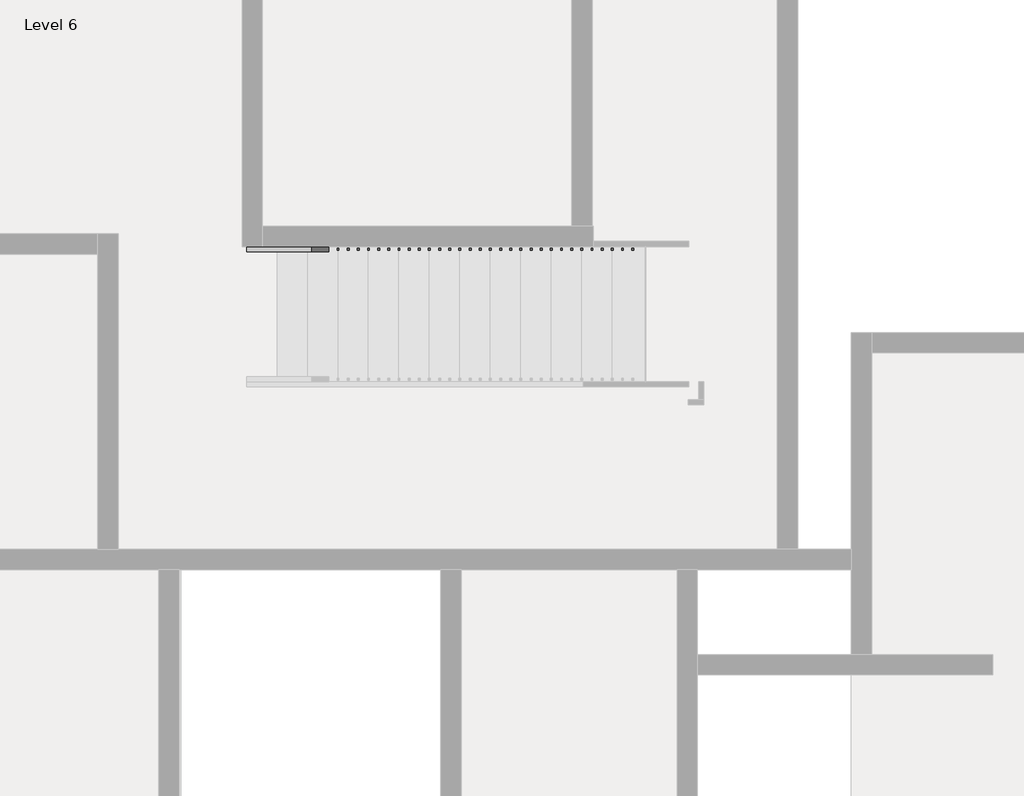
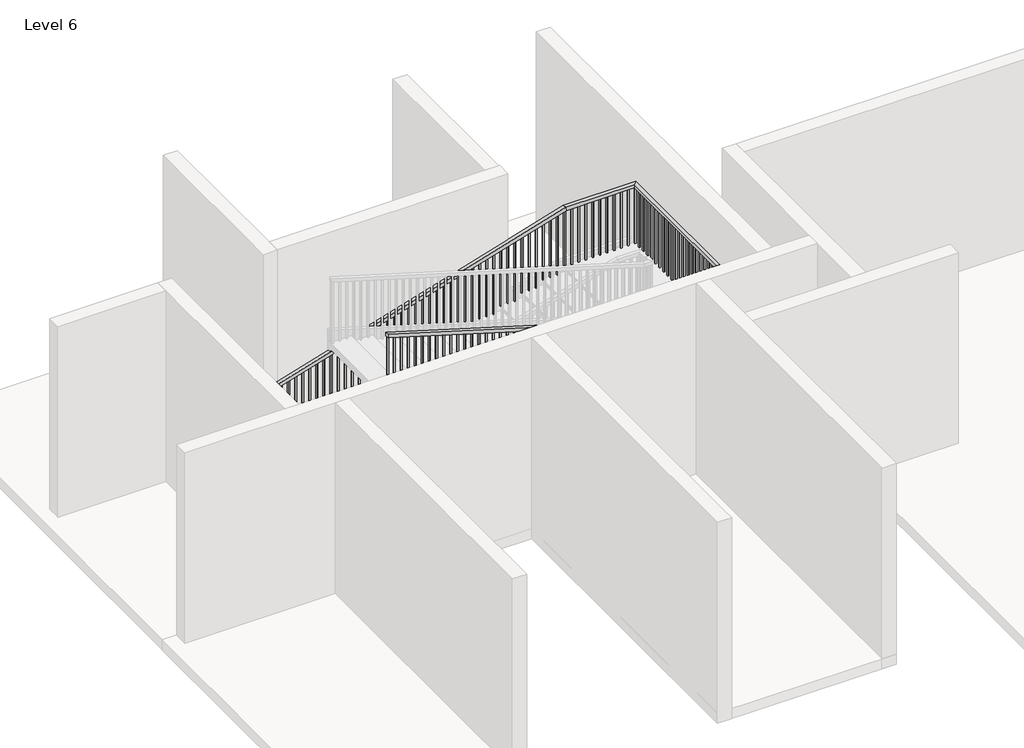
# One storey, part 10 of 14: 1 railing.
"""IFC4 building model written with IfcOpenShell, lengths in millimetres."""

from ifc_helpers import new_model, si_unit, frame, origin, place, context, project, spatial, polyline, outline, extrude, faceted_brep, element, save

model = new_model("IFC4")

# Units and contexts
model_context = context("Model", 3, world=origin())
ifc_project = project(units=[si_unit("LENGTHUNIT", "METRE", prefix="MILLI")], contexts=[model_context])

# Site, building, storey
site = spatial("IfcSite", under=ifc_project)
building = spatial("IfcBuilding", under=site)
storey = spatial("IfcBuildingStorey", under=building, Name="Level 6", Elevation=15240.0)

# Railing
placement = place(None, origin())
element("IfcRailing", 1, ObjectType="Handrail - Rectangular", at=placement, inside=storey, context=model_context, shape_type="SolidModel", body=[
    faceted_brep([(-5254.0891351, 12506.0715905, 16245.84), (-5254.0891351, 12506.0715905, 16192.8032429), (-5254.0891351, 12455.2715905, 16192.8032429), (-5254.0891351, 12455.2715905, 16245.84), (-986.8891351, 12506.0715905, 17526.0), (-979.4332782, 12506.0715905, 17475.2), (-979.4332782, 12455.2715905, 17475.2), (-986.8891351, 12455.2715905, 17526.0), (54.5108649, 12506.0715905, 17526.0), (54.5108649, 12506.0715905, 17475.2), (3.7108649, 12455.2715905, 17475.2), (3.7108649, 12455.2715905, 17526.0), (54.5108649, 9478.4949943, 17526.0), (54.5108649, 9478.4949943, 17475.2), (3.7108649, 9529.2949943, 17475.2), (3.7108649, 9529.2949943, 17526.0), (-682.0891351, 9478.4949943, 17526.0), (-689.544992, 9478.4949943, 17475.2), (-689.544992, 9529.2949943, 17475.2), (-682.0891351, 9529.2949943, 17526.0), (-5254.0891351, 9478.4949943, 18897.6), (-5254.0891351, 9529.2949943, 18897.6), (-5254.0891351, 9529.2949943, 18844.5632429), (-5254.0891351, 9478.4949943, 18844.5632429)], [[[0, 1, 2, 3]], [[1, 0, 4, 5]], [[2, 1, 5, 6]], [[3, 2, 6, 7]], [[0, 3, 7, 4]], [[5, 4, 8, 9]], [[6, 5, 9, 10]], [[7, 6, 10, 11]], [[4, 7, 11, 8]], [[9, 8, 12, 13]], [[10, 9, 13, 14]], [[11, 10, 14, 15]], [[8, 11, 15, 12]], [[13, 12, 16, 17]], [[14, 13, 17, 18]], [[15, 14, 18, 19]], [[12, 15, 19, 16]], [[20, 21, 22, 23]], [[17, 16, 20, 23]], [[18, 17, 23, 22]], [[19, 18, 22, 21]], [[16, 19, 21, 20]]]),
    extrude(outline(polyline([(18816.9407429, -5162.0141351), (17891.76, -5162.0141351), (17891.76, -5142.9641351), (18811.2257429, -5142.9641351), (18816.9407429, -5162.0141351)])), frame((0.0, 9494.3699943, 0.0), z_axis=(0.0, 1.0, 0.0), x_axis=(0.0, 0.0, 1.0)), (0.0, 0.0, 1.0), 19.05),
    extrude(outline(polyline([(18786.4607429, -5060.4141351), (17891.76, -5060.4141351), (17891.76, -5041.3641351), (18780.7457429, -5041.3641351), (18786.4607429, -5060.4141351)])), frame((0.0, 9494.3699943, 0.0), z_axis=(0.0, 1.0, 0.0), x_axis=(0.0, 0.0, 1.0)), (0.0, 0.0, 1.0), 19.05),
    extrude(outline(polyline([(18755.9807429, -4958.8141351), (17891.76, -4958.8141351), (17891.76, -4939.7641351), (18750.2657429, -4939.7641351), (18755.9807429, -4958.8141351)])), frame((0.0, 9494.3699943, 0.0), z_axis=(0.0, 1.0, 0.0), x_axis=(0.0, 0.0, 1.0)), (0.0, 0.0, 1.0), 19.05),
    extrude(outline(polyline([(18725.5007429, -4857.2141351), (17800.32, -4857.2141351), (17800.32, -4838.1641351), (18719.7857429, -4838.1641351), (18725.5007429, -4857.2141351)])), frame((0.0, 9494.3699943, 0.0), z_axis=(0.0, 1.0, 0.0), x_axis=(0.0, 0.0, 1.0)), (0.0, 0.0, 1.0), 19.05),
    extrude(outline(polyline([(18695.0207429, -4755.6141351), (17800.32, -4755.6141351), (17800.32, -4736.5641351), (18689.3057429, -4736.5641351), (18695.0207429, -4755.6141351)])), frame((0.0, 9494.3699943, 0.0), z_axis=(0.0, 1.0, 0.0), x_axis=(0.0, 0.0, 1.0)), (0.0, 0.0, 1.0), 19.05),
    extrude(outline(polyline([(18664.5407429, -4654.0141351), (17800.32, -4654.0141351), (17800.32, -4634.9641351), (18658.8257429, -4634.9641351), (18664.5407429, -4654.0141351)])), frame((0.0, 9494.3699943, 0.0), z_axis=(0.0, 1.0, 0.0), x_axis=(0.0, 0.0, 1.0)), (0.0, 0.0, 1.0), 19.05),
    extrude(outline(polyline([(18634.0607429, -4552.4141351), (17708.88, -4552.4141351), (17708.88, -4533.3641351), (18628.3457429, -4533.3641351), (18634.0607429, -4552.4141351)])), frame((0.0, 9494.3699943, 0.0), z_axis=(0.0, 1.0, 0.0), x_axis=(0.0, 0.0, 1.0)), (0.0, 0.0, 1.0), 19.05),
    extrude(outline(polyline([(18603.5807429, -4450.8141351), (17708.88, -4450.8141351), (17708.88, -4431.7641351), (18597.8657429, -4431.7641351), (18603.5807429, -4450.8141351)])), frame((0.0, 9494.3699943, 0.0), z_axis=(0.0, 1.0, 0.0), x_axis=(0.0, 0.0, 1.0)), (0.0, 0.0, 1.0), 19.05),
    extrude(outline(polyline([(18573.1007429, -4349.2141351), (17708.88, -4349.2141351), (17708.88, -4330.1641351), (18567.3857429, -4330.1641351), (18573.1007429, -4349.2141351)])), frame((0.0, 9494.3699943, 0.0), z_axis=(0.0, 1.0, 0.0), x_axis=(0.0, 0.0, 1.0)), (0.0, 0.0, 1.0), 19.05),
    extrude(outline(polyline([(18542.6207429, -4247.6141351), (17617.44, -4247.6141351), (17617.44, -4228.5641351), (18536.9057429, -4228.5641351), (18542.6207429, -4247.6141351)])), frame((0.0, 9494.3699943, 0.0), z_axis=(0.0, 1.0, 0.0), x_axis=(0.0, 0.0, 1.0)), (0.0, 0.0, 1.0), 19.05),
    extrude(outline(polyline([(18512.1407429, -4146.0141351), (17617.44, -4146.0141351), (17617.44, -4126.9641351), (18506.4257429, -4126.9641351), (18512.1407429, -4146.0141351)])), frame((0.0, 9494.3699943, 0.0), z_axis=(0.0, 1.0, 0.0), x_axis=(0.0, 0.0, 1.0)), (0.0, 0.0, 1.0), 19.05),
    extrude(outline(polyline([(18481.6607429, -4044.4141351), (17617.44, -4044.4141351), (17617.44, -4025.3641351), (18475.9457429, -4025.3641351), (18481.6607429, -4044.4141351)])), frame((0.0, 9494.3699943, 0.0), z_axis=(0.0, 1.0, 0.0), x_axis=(0.0, 0.0, 1.0)), (0.0, 0.0, 1.0), 19.05),
    extrude(outline(polyline([(18451.1807429, -3942.8141351), (17526.0, -3942.8141351), (17526.0, -3923.7641351), (18445.4657429, -3923.7641351), (18451.1807429, -3942.8141351)])), frame((0.0, 9494.3699943, 0.0), z_axis=(0.0, 1.0, 0.0), x_axis=(0.0, 0.0, 1.0)), (0.0, 0.0, 1.0), 19.05),
    extrude(outline(polyline([(18420.7007429, -3841.2141351), (17526.0, -3841.2141351), (17526.0, -3822.1641351), (18414.9857429, -3822.1641351), (18420.7007429, -3841.2141351)])), frame((0.0, 9494.3699943, 0.0), z_axis=(0.0, 1.0, 0.0), x_axis=(0.0, 0.0, 1.0)), (0.0, 0.0, 1.0), 19.05),
    extrude(outline(polyline([(18390.2207429, -3739.6141351), (17526.0, -3739.6141351), (17526.0, -3720.5641351), (18384.5057429, -3720.5641351), (18390.2207429, -3739.6141351)])), frame((0.0, 9494.3699943, 0.0), z_axis=(0.0, 1.0, 0.0), x_axis=(0.0, 0.0, 1.0)), (0.0, 0.0, 1.0), 19.05),
    extrude(outline(polyline([(18359.7407429, -3638.0141351), (17434.56, -3638.0141351), (17434.56, -3618.9641351), (18354.0257429, -3618.9641351), (18359.7407429, -3638.0141351)])), frame((0.0, 9494.3699943, 0.0), z_axis=(0.0, 1.0, 0.0), x_axis=(0.0, 0.0, 1.0)), (0.0, 0.0, 1.0), 19.05),
    extrude(outline(polyline([(18329.2607429, -3536.4141351), (17434.56, -3536.4141351), (17434.56, -3517.3641351), (18323.5457429, -3517.3641351), (18329.2607429, -3536.4141351)])), frame((0.0, 9494.3699943, 0.0), z_axis=(0.0, 1.0, 0.0), x_axis=(0.0, 0.0, 1.0)), (0.0, 0.0, 1.0), 19.05),
    extrude(outline(polyline([(18298.7807429, -3434.8141351), (17434.56, -3434.8141351), (17434.56, -3415.7641351), (18293.0657429, -3415.7641351), (18298.7807429, -3434.8141351)])), frame((0.0, 9494.3699943, 0.0), z_axis=(0.0, 1.0, 0.0), x_axis=(0.0, 0.0, 1.0)), (0.0, 0.0, 1.0), 19.05),
    extrude(outline(polyline([(18268.3007429, -3333.2141351), (17343.12, -3333.2141351), (17343.12, -3314.1641351), (18262.5857429, -3314.1641351), (18268.3007429, -3333.2141351)])), frame((0.0, 9494.3699943, 0.0), z_axis=(0.0, 1.0, 0.0), x_axis=(0.0, 0.0, 1.0)), (0.0, 0.0, 1.0), 19.05),
    extrude(outline(polyline([(18237.8207429, -3231.6141351), (17343.12, -3231.6141351), (17343.12, -3212.5641351), (18232.1057429, -3212.5641351), (18237.8207429, -3231.6141351)])), frame((0.0, 9494.3699943, 0.0), z_axis=(0.0, 1.0, 0.0), x_axis=(0.0, 0.0, 1.0)), (0.0, 0.0, 1.0), 19.05),
    extrude(outline(polyline([(18207.3407429, -3130.0141351), (17343.12, -3130.0141351), (17343.12, -3110.9641351), (18201.6257429, -3110.9641351), (18207.3407429, -3130.0141351)])), frame((0.0, 9494.3699943, 0.0), z_axis=(0.0, 1.0, 0.0), x_axis=(0.0, 0.0, 1.0)), (0.0, 0.0, 1.0), 19.05),
    extrude(outline(polyline([(18176.8607429, -3028.4141351), (17251.68, -3028.4141351), (17251.68, -3009.3641351), (18171.1457429, -3009.3641351), (18176.8607429, -3028.4141351)])), frame((0.0, 9494.3699943, 0.0), z_axis=(0.0, 1.0, 0.0), x_axis=(0.0, 0.0, 1.0)), (0.0, 0.0, 1.0), 19.05),
    extrude(outline(polyline([(18146.3807429, -2926.8141351), (17251.68, -2926.8141351), (17251.68, -2907.7641351), (18140.6657429, -2907.7641351), (18146.3807429, -2926.8141351)])), frame((0.0, 9494.3699943, 0.0), z_axis=(0.0, 1.0, 0.0), x_axis=(0.0, 0.0, 1.0)), (0.0, 0.0, 1.0), 19.05),
    extrude(outline(polyline([(18115.9007429, -2825.2141351), (17251.68, -2825.2141351), (17251.68, -2806.1641351), (18110.1857429, -2806.1641351), (18115.9007429, -2825.2141351)])), frame((0.0, 9494.3699943, 0.0), z_axis=(0.0, 1.0, 0.0), x_axis=(0.0, 0.0, 1.0)), (0.0, 0.0, 1.0), 19.05),
    extrude(outline(polyline([(18085.4207429, -2723.6141351), (17160.24, -2723.6141351), (17160.24, -2704.5641351), (18079.7057429, -2704.5641351), (18085.4207429, -2723.6141351)])), frame((0.0, 9494.3699943, 0.0), z_axis=(0.0, 1.0, 0.0), x_axis=(0.0, 0.0, 1.0)), (0.0, 0.0, 1.0), 19.05),
    extrude(outline(polyline([(18054.9407429, -2622.0141351), (17160.24, -2622.0141351), (17160.24, -2602.9641351), (18049.2257429, -2602.9641351), (18054.9407429, -2622.0141351)])), frame((0.0, 9494.3699943, 0.0), z_axis=(0.0, 1.0, 0.0), x_axis=(0.0, 0.0, 1.0)), (0.0, 0.0, 1.0), 19.05),
    extrude(outline(polyline([(18024.4607429, -2520.4141351), (17160.24, -2520.4141351), (17160.24, -2501.3641351), (18018.7457429, -2501.3641351), (18024.4607429, -2520.4141351)])), frame((0.0, 9494.3699943, 0.0), z_axis=(0.0, 1.0, 0.0), x_axis=(0.0, 0.0, 1.0)), (0.0, 0.0, 1.0), 19.05),
    extrude(outline(polyline([(17993.9807429, -2418.8141351), (17068.8, -2418.8141351), (17068.8, -2399.7641351), (17988.2657429, -2399.7641351), (17993.9807429, -2418.8141351)])), frame((0.0, 9494.3699943, 0.0), z_axis=(0.0, 1.0, 0.0), x_axis=(0.0, 0.0, 1.0)), (0.0, 0.0, 1.0), 19.05),
    extrude(outline(polyline([(17963.5007429, -2317.2141351), (17068.8, -2317.2141351), (17068.8, -2298.1641351), (17957.7857429, -2298.1641351), (17963.5007429, -2317.2141351)])), frame((0.0, 9494.3699943, 0.0), z_axis=(0.0, 1.0, 0.0), x_axis=(0.0, 0.0, 1.0)), (0.0, 0.0, 1.0), 19.05),
    extrude(outline(polyline([(17933.0207429, -2215.6141351), (17068.8, -2215.6141351), (17068.8, -2196.5641351), (17927.3057429, -2196.5641351), (17933.0207429, -2215.6141351)])), frame((0.0, 9494.3699943, 0.0), z_axis=(0.0, 1.0, 0.0), x_axis=(0.0, 0.0, 1.0)), (0.0, 0.0, 1.0), 19.05),
    extrude(outline(polyline([(17902.5407429, -2114.0141351), (16977.36, -2114.0141351), (16977.36, -2094.9641351), (17896.8257429, -2094.9641351), (17902.5407429, -2114.0141351)])), frame((0.0, 9494.3699943, 0.0), z_axis=(0.0, 1.0, 0.0), x_axis=(0.0, 0.0, 1.0)), (0.0, 0.0, 1.0), 19.05),
    extrude(outline(polyline([(17872.0607429, -2012.4141351), (16977.36, -2012.4141351), (16977.36, -1993.3641351), (17866.3457429, -1993.3641351), (17872.0607429, -2012.4141351)])), frame((0.0, 9494.3699943, 0.0), z_axis=(0.0, 1.0, 0.0), x_axis=(0.0, 0.0, 1.0)), (0.0, 0.0, 1.0), 19.05),
    extrude(outline(polyline([(17841.5807429, -1910.8141351), (16977.36, -1910.8141351), (16977.36, -1891.7641351), (17835.8657429, -1891.7641351), (17841.5807429, -1910.8141351)])), frame((0.0, 9494.3699943, 0.0), z_axis=(0.0, 1.0, 0.0), x_axis=(0.0, 0.0, 1.0)), (0.0, 0.0, 1.0), 19.05),
    extrude(outline(polyline([(17811.1007429, -1809.2141351), (16885.92, -1809.2141351), (16885.92, -1790.1641351), (17805.3857429, -1790.1641351), (17811.1007429, -1809.2141351)])), frame((0.0, 9494.3699943, 0.0), z_axis=(0.0, 1.0, 0.0), x_axis=(0.0, 0.0, 1.0)), (0.0, 0.0, 1.0), 19.05),
    extrude(outline(polyline([(17780.6207429, -1707.6141351), (16885.92, -1707.6141351), (16885.92, -1688.5641351), (17774.9057429, -1688.5641351), (17780.6207429, -1707.6141351)])), frame((0.0, 9494.3699943, 0.0), z_axis=(0.0, 1.0, 0.0), x_axis=(0.0, 0.0, 1.0)), (0.0, 0.0, 1.0), 19.05),
    extrude(outline(polyline([(17750.1407429, -1606.0141351), (16885.92, -1606.0141351), (16885.92, -1586.9641351), (17744.4257429, -1586.9641351), (17750.1407429, -1606.0141351)])), frame((0.0, 9494.3699943, 0.0), z_axis=(0.0, 1.0, 0.0), x_axis=(0.0, 0.0, 1.0)), (0.0, 0.0, 1.0), 19.05),
    extrude(outline(polyline([(17719.6607429, -1504.4141351), (16794.48, -1504.4141351), (16794.48, -1485.3641351), (17713.9457429, -1485.3641351), (17719.6607429, -1504.4141351)])), frame((0.0, 9494.3699943, 0.0), z_axis=(0.0, 1.0, 0.0), x_axis=(0.0, 0.0, 1.0)), (0.0, 0.0, 1.0), 19.05),
    extrude(outline(polyline([(17689.1807429, -1402.8141351), (16794.48, -1402.8141351), (16794.48, -1383.7641351), (17683.4657429, -1383.7641351), (17689.1807429, -1402.8141351)])), frame((0.0, 9494.3699943, 0.0), z_axis=(0.0, 1.0, 0.0), x_axis=(0.0, 0.0, 1.0)), (0.0, 0.0, 1.0), 19.05),
    extrude(outline(polyline([(17658.7007429, -1301.2141351), (16794.48, -1301.2141351), (16794.48, -1282.1641351), (17652.9857429, -1282.1641351), (17658.7007429, -1301.2141351)])), frame((0.0, 9494.3699943, 0.0), z_axis=(0.0, 1.0, 0.0), x_axis=(0.0, 0.0, 1.0)), (0.0, 0.0, 1.0), 19.05),
    extrude(outline(polyline([(17628.2207429, -1199.6141351), (16703.04, -1199.6141351), (16703.04, -1180.5641351), (17622.5057429, -1180.5641351), (17628.2207429, -1199.6141351)])), frame((0.0, 9494.3699943, 0.0), z_axis=(0.0, 1.0, 0.0), x_axis=(0.0, 0.0, 1.0)), (0.0, 0.0, 1.0), 19.05),
    extrude(outline(polyline([(17597.7407429, -1098.0141351), (16703.04, -1098.0141351), (16703.04, -1078.9641351), (17592.0257429, -1078.9641351), (17597.7407429, -1098.0141351)])), frame((0.0, 9494.3699943, 0.0), z_axis=(0.0, 1.0, 0.0), x_axis=(0.0, 0.0, 1.0)), (0.0, 0.0, 1.0), 19.05),
    extrude(outline(polyline([(17567.2607429, -996.4141351), (16703.04, -996.4141351), (16703.04, -977.3641351), (17561.5457429, -977.3641351), (17567.2607429, -996.4141351)])), frame((0.0, 9494.3699943, 0.0), z_axis=(0.0, 1.0, 0.0), x_axis=(0.0, 0.0, 1.0)), (0.0, 0.0, 1.0), 19.05),
    extrude(outline(polyline([(17536.7807429, -894.8141351), (16611.6, -894.8141351), (16611.6, -875.7641351), (17531.0657429, -875.7641351), (17536.7807429, -894.8141351)])), frame((0.0, 9494.3699943, 0.0), z_axis=(0.0, 1.0, 0.0), x_axis=(0.0, 0.0, 1.0)), (0.0, 0.0, 1.0), 19.05),
    extrude(outline(polyline([(17506.3007429, -793.2141351), (16611.6, -793.2141351), (16611.6, -774.1641351), (17500.5857429, -774.1641351), (17506.3007429, -793.2141351)])), frame((0.0, 9494.3699943, 0.0), z_axis=(0.0, 1.0, 0.0), x_axis=(0.0, 0.0, 1.0)), (0.0, 0.0, 1.0), 19.05),
    extrude(outline(polyline([(-672.5641351, 9494.3699943), (-691.6141351, 9494.3699943), (-691.6141351, 9513.4199943), (-672.5641351, 9513.4199943), (-672.5641351, 9494.3699943)])), frame((0.0, 0.0, 16611.6), z_axis=(0.0, 0.0, 1.0), x_axis=(1.0, 0.0, 0.0)), (0.0, 0.0, 1.0), 863.6),
    extrude(outline(polyline([(-570.9641351, 9494.3699943), (-590.0141351, 9494.3699943), (-590.0141351, 9513.4199943), (-570.9641351, 9513.4199943), (-570.9641351, 9494.3699943)])), frame((0.0, 0.0, 16611.6), z_axis=(0.0, 0.0, 1.0), x_axis=(1.0, 0.0, 0.0)), (0.0, 0.0, 1.0), 863.6),
    extrude(outline(polyline([(-469.3641351, 9494.3699943), (-488.4141351, 9494.3699943), (-488.4141351, 9513.4199943), (-469.3641351, 9513.4199943), (-469.3641351, 9494.3699943)])), frame((0.0, 0.0, 16611.6), z_axis=(0.0, 0.0, 1.0), x_axis=(1.0, 0.0, 0.0)), (0.0, 0.0, 1.0), 863.6),
    extrude(outline(polyline([(-367.7641351, 9494.3699943), (-386.8141351, 9494.3699943), (-386.8141351, 9513.4199943), (-367.7641351, 9513.4199943), (-367.7641351, 9494.3699943)])), frame((0.0, 0.0, 16611.6), z_axis=(0.0, 0.0, 1.0), x_axis=(1.0, 0.0, 0.0)), (0.0, 0.0, 1.0), 863.6),
    extrude(outline(polyline([(-266.1641351, 9494.3699943), (-285.2141351, 9494.3699943), (-285.2141351, 9513.4199943), (-266.1641351, 9513.4199943), (-266.1641351, 9494.3699943)])), frame((0.0, 0.0, 16611.6), z_axis=(0.0, 0.0, 1.0), x_axis=(1.0, 0.0, 0.0)), (0.0, 0.0, 1.0), 863.6),
    extrude(outline(polyline([(-164.5641351, 9494.3699943), (-183.6141351, 9494.3699943), (-183.6141351, 9513.4199943), (-164.5641351, 9513.4199943), (-164.5641351, 9494.3699943)])), frame((0.0, 0.0, 16611.6), z_axis=(0.0, 0.0, 1.0), x_axis=(1.0, 0.0, 0.0)), (0.0, 0.0, 1.0), 863.6),
    extrude(outline(polyline([(-62.9641351, 9494.3699943), (-82.0141351, 9494.3699943), (-82.0141351, 9513.4199943), (-62.9641351, 9513.4199943), (-62.9641351, 9494.3699943)])), frame((0.0, 0.0, 16611.6), z_axis=(0.0, 0.0, 1.0), x_axis=(1.0, 0.0, 0.0)), (0.0, 0.0, 1.0), 863.6),
    extrude(outline(polyline([(38.6358649, 9543.7965905), (38.6358649, 9524.7465905), (19.5858649, 9524.7465905), (19.5858649, 9543.7965905), (38.6358649, 9543.7965905)])), frame((0.0, 0.0, 16611.6), z_axis=(0.0, 0.0, 1.0), x_axis=(1.0, 0.0, 0.0)), (0.0, 0.0, 1.0), 863.6),
    extrude(outline(polyline([(38.6358649, 9645.3965905), (38.6358649, 9626.3465905), (19.5858649, 9626.3465905), (19.5858649, 9645.3965905), (38.6358649, 9645.3965905)])), frame((0.0, 0.0, 16611.6), z_axis=(0.0, 0.0, 1.0), x_axis=(1.0, 0.0, 0.0)), (0.0, 0.0, 1.0), 863.6),
    extrude(outline(polyline([(38.6358649, 9746.9965905), (38.6358649, 9727.9465905), (19.5858649, 9727.9465905), (19.5858649, 9746.9965905), (38.6358649, 9746.9965905)])), frame((0.0, 0.0, 16611.6), z_axis=(0.0, 0.0, 1.0), x_axis=(1.0, 0.0, 0.0)), (0.0, 0.0, 1.0), 863.6),
    extrude(outline(polyline([(38.6358649, 9848.5965905), (38.6358649, 9829.5465905), (19.5858649, 9829.5465905), (19.5858649, 9848.5965905), (38.6358649, 9848.5965905)])), frame((0.0, 0.0, 16611.6), z_axis=(0.0, 0.0, 1.0), x_axis=(1.0, 0.0, 0.0)), (0.0, 0.0, 1.0), 863.6),
    extrude(outline(polyline([(38.6358649, 9950.1965905), (38.6358649, 9931.1465905), (19.5858649, 9931.1465905), (19.5858649, 9950.1965905), (38.6358649, 9950.1965905)])), frame((0.0, 0.0, 16611.6), z_axis=(0.0, 0.0, 1.0), x_axis=(1.0, 0.0, 0.0)), (0.0, 0.0, 1.0), 863.6),
    extrude(outline(polyline([(38.6358649, 10051.7965905), (38.6358649, 10032.7465905), (19.5858649, 10032.7465905), (19.5858649, 10051.7965905), (38.6358649, 10051.7965905)])), frame((0.0, 0.0, 16611.6), z_axis=(0.0, 0.0, 1.0), x_axis=(1.0, 0.0, 0.0)), (0.0, 0.0, 1.0), 863.6),
    extrude(outline(polyline([(38.6358649, 10153.3965905), (38.6358649, 10134.3465905), (19.5858649, 10134.3465905), (19.5858649, 10153.3965905), (38.6358649, 10153.3965905)])), frame((0.0, 0.0, 16611.6), z_axis=(0.0, 0.0, 1.0), x_axis=(1.0, 0.0, 0.0)), (0.0, 0.0, 1.0), 863.6),
    extrude(outline(polyline([(38.6358649, 10254.9965905), (38.6358649, 10235.9465905), (19.5858649, 10235.9465905), (19.5858649, 10254.9965905), (38.6358649, 10254.9965905)])), frame((0.0, 0.0, 16611.6), z_axis=(0.0, 0.0, 1.0), x_axis=(1.0, 0.0, 0.0)), (0.0, 0.0, 1.0), 863.6),
    extrude(outline(polyline([(38.6358649, 10356.5965905), (38.6358649, 10337.5465905), (19.5858649, 10337.5465905), (19.5858649, 10356.5965905), (38.6358649, 10356.5965905)])), frame((0.0, 0.0, 16611.6), z_axis=(0.0, 0.0, 1.0), x_axis=(1.0, 0.0, 0.0)), (0.0, 0.0, 1.0), 863.6),
    extrude(outline(polyline([(38.6358649, 10458.1965905), (38.6358649, 10439.1465905), (19.5858649, 10439.1465905), (19.5858649, 10458.1965905), (38.6358649, 10458.1965905)])), frame((0.0, 0.0, 16611.6), z_axis=(0.0, 0.0, 1.0), x_axis=(1.0, 0.0, 0.0)), (0.0, 0.0, 1.0), 863.6),
    extrude(outline(polyline([(38.6358649, 10559.7965905), (38.6358649, 10540.7465905), (19.5858649, 10540.7465905), (19.5858649, 10559.7965905), (38.6358649, 10559.7965905)])), frame((0.0, 0.0, 16611.6), z_axis=(0.0, 0.0, 1.0), x_axis=(1.0, 0.0, 0.0)), (0.0, 0.0, 1.0), 863.6),
    extrude(outline(polyline([(38.6358649, 10661.3965905), (38.6358649, 10642.3465905), (19.5858649, 10642.3465905), (19.5858649, 10661.3965905), (38.6358649, 10661.3965905)])), frame((0.0, 0.0, 16611.6), z_axis=(0.0, 0.0, 1.0), x_axis=(1.0, 0.0, 0.0)), (0.0, 0.0, 1.0), 863.6),
    extrude(outline(polyline([(38.6358649, 10762.9965905), (38.6358649, 10743.9465905), (19.5858649, 10743.9465905), (19.5858649, 10762.9965905), (38.6358649, 10762.9965905)])), frame((0.0, 0.0, 16611.6), z_axis=(0.0, 0.0, 1.0), x_axis=(1.0, 0.0, 0.0)), (0.0, 0.0, 1.0), 863.6),
    extrude(outline(polyline([(38.6358649, 10864.5965905), (38.6358649, 10845.5465905), (19.5858649, 10845.5465905), (19.5858649, 10864.5965905), (38.6358649, 10864.5965905)])), frame((0.0, 0.0, 16611.6), z_axis=(0.0, 0.0, 1.0), x_axis=(1.0, 0.0, 0.0)), (0.0, 0.0, 1.0), 863.6),
    extrude(outline(polyline([(38.6358649, 10966.1965905), (38.6358649, 10947.1465905), (19.5858649, 10947.1465905), (19.5858649, 10966.1965905), (38.6358649, 10966.1965905)])), frame((0.0, 0.0, 16611.6), z_axis=(0.0, 0.0, 1.0), x_axis=(1.0, 0.0, 0.0)), (0.0, 0.0, 1.0), 863.6),
    extrude(outline(polyline([(38.6358649, 11067.7965905), (38.6358649, 11048.7465905), (19.5858649, 11048.7465905), (19.5858649, 11067.7965905), (38.6358649, 11067.7965905)])), frame((0.0, 0.0, 16611.6), z_axis=(0.0, 0.0, 1.0), x_axis=(1.0, 0.0, 0.0)), (0.0, 0.0, 1.0), 863.6),
    extrude(outline(polyline([(38.6358649, 11169.3965905), (38.6358649, 11150.3465905), (19.5858649, 11150.3465905), (19.5858649, 11169.3965905), (38.6358649, 11169.3965905)])), frame((0.0, 0.0, 16611.6), z_axis=(0.0, 0.0, 1.0), x_axis=(1.0, 0.0, 0.0)), (0.0, 0.0, 1.0), 863.6),
    extrude(outline(polyline([(38.6358649, 11270.9965905), (38.6358649, 11251.9465905), (19.5858649, 11251.9465905), (19.5858649, 11270.9965905), (38.6358649, 11270.9965905)])), frame((0.0, 0.0, 16611.6), z_axis=(0.0, 0.0, 1.0), x_axis=(1.0, 0.0, 0.0)), (0.0, 0.0, 1.0), 863.6),
    extrude(outline(polyline([(38.6358649, 11372.5965905), (38.6358649, 11353.5465905), (19.5858649, 11353.5465905), (19.5858649, 11372.5965905), (38.6358649, 11372.5965905)])), frame((0.0, 0.0, 16611.6), z_axis=(0.0, 0.0, 1.0), x_axis=(1.0, 0.0, 0.0)), (0.0, 0.0, 1.0), 863.6),
    extrude(outline(polyline([(38.6358649, 11474.1965905), (38.6358649, 11455.1465905), (19.5858649, 11455.1465905), (19.5858649, 11474.1965905), (38.6358649, 11474.1965905)])), frame((0.0, 0.0, 16611.6), z_axis=(0.0, 0.0, 1.0), x_axis=(1.0, 0.0, 0.0)), (0.0, 0.0, 1.0), 863.6),
    extrude(outline(polyline([(38.6358649, 11575.7965905), (38.6358649, 11556.7465905), (19.5858649, 11556.7465905), (19.5858649, 11575.7965905), (38.6358649, 11575.7965905)])), frame((0.0, 0.0, 16611.6), z_axis=(0.0, 0.0, 1.0), x_axis=(1.0, 0.0, 0.0)), (0.0, 0.0, 1.0), 863.6),
    extrude(outline(polyline([(38.6358649, 11677.3965905), (38.6358649, 11658.3465905), (19.5858649, 11658.3465905), (19.5858649, 11677.3965905), (38.6358649, 11677.3965905)])), frame((0.0, 0.0, 16611.6), z_axis=(0.0, 0.0, 1.0), x_axis=(1.0, 0.0, 0.0)), (0.0, 0.0, 1.0), 863.6),
    extrude(outline(polyline([(38.6358649, 11778.9965905), (38.6358649, 11759.9465905), (19.5858649, 11759.9465905), (19.5858649, 11778.9965905), (38.6358649, 11778.9965905)])), frame((0.0, 0.0, 16611.6), z_axis=(0.0, 0.0, 1.0), x_axis=(1.0, 0.0, 0.0)), (0.0, 0.0, 1.0), 863.6),
    extrude(outline(polyline([(38.6358649, 11880.5965905), (38.6358649, 11861.5465905), (19.5858649, 11861.5465905), (19.5858649, 11880.5965905), (38.6358649, 11880.5965905)])), frame((0.0, 0.0, 16611.6), z_axis=(0.0, 0.0, 1.0), x_axis=(1.0, 0.0, 0.0)), (0.0, 0.0, 1.0), 863.6),
    extrude(outline(polyline([(38.6358649, 11982.1965905), (38.6358649, 11963.1465905), (19.5858649, 11963.1465905), (19.5858649, 11982.1965905), (38.6358649, 11982.1965905)])), frame((0.0, 0.0, 16611.6), z_axis=(0.0, 0.0, 1.0), x_axis=(1.0, 0.0, 0.0)), (0.0, 0.0, 1.0), 863.6),
    extrude(outline(polyline([(38.6358649, 12083.7965905), (38.6358649, 12064.7465905), (19.5858649, 12064.7465905), (19.5858649, 12083.7965905), (38.6358649, 12083.7965905)])), frame((0.0, 0.0, 16611.6), z_axis=(0.0, 0.0, 1.0), x_axis=(1.0, 0.0, 0.0)), (0.0, 0.0, 1.0), 863.6),
    extrude(outline(polyline([(38.6358649, 12185.3965905), (38.6358649, 12166.3465905), (19.5858649, 12166.3465905), (19.5858649, 12185.3965905), (38.6358649, 12185.3965905)])), frame((0.0, 0.0, 16611.6), z_axis=(0.0, 0.0, 1.0), x_axis=(1.0, 0.0, 0.0)), (0.0, 0.0, 1.0), 863.6),
    extrude(outline(polyline([(38.6358649, 12286.9965905), (38.6358649, 12267.9465905), (19.5858649, 12267.9465905), (19.5858649, 12286.9965905), (38.6358649, 12286.9965905)])), frame((0.0, 0.0, 16611.6), z_axis=(0.0, 0.0, 1.0), x_axis=(1.0, 0.0, 0.0)), (0.0, 0.0, 1.0), 863.6),
    extrude(outline(polyline([(38.6358649, 12388.5965905), (38.6358649, 12369.5465905), (19.5858649, 12369.5465905), (19.5858649, 12388.5965905), (38.6358649, 12388.5965905)])), frame((0.0, 0.0, 16611.6), z_axis=(0.0, 0.0, 1.0), x_axis=(1.0, 0.0, 0.0)), (0.0, 0.0, 1.0), 863.6),
    extrude(outline(polyline([(-82.0141351, 12490.1965905), (-62.9641351, 12490.1965905), (-62.9641351, 12471.1465905), (-82.0141351, 12471.1465905), (-82.0141351, 12490.1965905)])), frame((0.0, 0.0, 16611.6), z_axis=(0.0, 0.0, 1.0), x_axis=(1.0, 0.0, 0.0)), (0.0, 0.0, 1.0), 863.6),
    extrude(outline(polyline([(-183.6141351, 12490.1965905), (-164.5641351, 12490.1965905), (-164.5641351, 12471.1465905), (-183.6141351, 12471.1465905), (-183.6141351, 12490.1965905)])), frame((0.0, 0.0, 16611.6), z_axis=(0.0, 0.0, 1.0), x_axis=(1.0, 0.0, 0.0)), (0.0, 0.0, 1.0), 863.6),
    extrude(outline(polyline([(-285.2141351, 12490.1965905), (-266.1641351, 12490.1965905), (-266.1641351, 12471.1465905), (-285.2141351, 12471.1465905), (-285.2141351, 12490.1965905)])), frame((0.0, 0.0, 16611.6), z_axis=(0.0, 0.0, 1.0), x_axis=(1.0, 0.0, 0.0)), (0.0, 0.0, 1.0), 863.6),
    extrude(outline(polyline([(-386.8141351, 12490.1965905), (-367.7641351, 12490.1965905), (-367.7641351, 12471.1465905), (-386.8141351, 12471.1465905), (-386.8141351, 12490.1965905)])), frame((0.0, 0.0, 16611.6), z_axis=(0.0, 0.0, 1.0), x_axis=(1.0, 0.0, 0.0)), (0.0, 0.0, 1.0), 863.6),
    extrude(outline(polyline([(-488.4141351, 12490.1965905), (-469.3641351, 12490.1965905), (-469.3641351, 12471.1465905), (-488.4141351, 12471.1465905), (-488.4141351, 12490.1965905)])), frame((0.0, 0.0, 16611.6), z_axis=(0.0, 0.0, 1.0), x_axis=(1.0, 0.0, 0.0)), (0.0, 0.0, 1.0), 863.6),
    extrude(outline(polyline([(-590.0141351, 12490.1965905), (-570.9641351, 12490.1965905), (-570.9641351, 12471.1465905), (-590.0141351, 12471.1465905), (-590.0141351, 12490.1965905)])), frame((0.0, 0.0, 16611.6), z_axis=(0.0, 0.0, 1.0), x_axis=(1.0, 0.0, 0.0)), (0.0, 0.0, 1.0), 863.6),
    extrude(outline(polyline([(-691.6141351, 12490.1965905), (-672.5641351, 12490.1965905), (-672.5641351, 12471.1465905), (-691.6141351, 12471.1465905), (-691.6141351, 12490.1965905)])), frame((0.0, 0.0, 16611.6), z_axis=(0.0, 0.0, 1.0), x_axis=(1.0, 0.0, 0.0)), (0.0, 0.0, 1.0), 863.6),
    extrude(outline(polyline([(-793.2141351, 12490.1965905), (-774.1641351, 12490.1965905), (-774.1641351, 12471.1465905), (-793.2141351, 12471.1465905), (-793.2141351, 12490.1965905)])), frame((0.0, 0.0, 16611.6), z_axis=(0.0, 0.0, 1.0), x_axis=(1.0, 0.0, 0.0)), (0.0, 0.0, 1.0), 863.6),
    extrude(outline(polyline([(-894.8141351, 12490.1965905), (-875.7641351, 12490.1965905), (-875.7641351, 12471.1465905), (-894.8141351, 12471.1465905), (-894.8141351, 12490.1965905)])), frame((0.0, 0.0, 16611.6), z_axis=(0.0, 0.0, 1.0), x_axis=(1.0, 0.0, 0.0)), (0.0, 0.0, 1.0), 863.6),
    extrude(outline(polyline([(17470.1057429, -996.4141351), (16611.6, -996.4141351), (16611.6, -977.3641351), (17475.8207429, -977.3641351), (17470.1057429, -996.4141351)])), frame((0.0, 12471.1465905, 0.0), z_axis=(0.0, 1.0, 0.0), x_axis=(0.0, 0.0, 1.0)), (0.0, 0.0, 1.0), 19.05),
    extrude(outline(polyline([(17439.6257429, -1098.0141351), (16520.16, -1098.0141351), (16520.16, -1078.9641351), (17445.3407429, -1078.9641351), (17439.6257429, -1098.0141351)])), frame((0.0, 12471.1465905, 0.0), z_axis=(0.0, 1.0, 0.0), x_axis=(0.0, 0.0, 1.0)), (0.0, 0.0, 1.0), 19.05),
    extrude(outline(polyline([(17409.1457429, -1199.6141351), (16520.16, -1199.6141351), (16520.16, -1180.5641351), (17414.8607429, -1180.5641351), (17409.1457429, -1199.6141351)])), frame((0.0, 12471.1465905, 0.0), z_axis=(0.0, 1.0, 0.0), x_axis=(0.0, 0.0, 1.0)), (0.0, 0.0, 1.0), 19.05),
    extrude(outline(polyline([(17378.6657429, -1301.2141351), (16520.16, -1301.2141351), (16520.16, -1282.1641351), (17384.3807429, -1282.1641351), (17378.6657429, -1301.2141351)])), frame((0.0, 12471.1465905, 0.0), z_axis=(0.0, 1.0, 0.0), x_axis=(0.0, 0.0, 1.0)), (0.0, 0.0, 1.0), 19.05),
    extrude(outline(polyline([(17348.1857429, -1402.8141351), (16428.72, -1402.8141351), (16428.72, -1383.7641351), (17353.9007429, -1383.7641351), (17348.1857429, -1402.8141351)])), frame((0.0, 12471.1465905, 0.0), z_axis=(0.0, 1.0, 0.0), x_axis=(0.0, 0.0, 1.0)), (0.0, 0.0, 1.0), 19.05),
    extrude(outline(polyline([(17317.7057429, -1504.4141351), (16428.72, -1504.4141351), (16428.72, -1485.3641351), (17323.4207429, -1485.3641351), (17317.7057429, -1504.4141351)])), frame((0.0, 12471.1465905, 0.0), z_axis=(0.0, 1.0, 0.0), x_axis=(0.0, 0.0, 1.0)), (0.0, 0.0, 1.0), 19.05),
    extrude(outline(polyline([(17287.2257429, -1606.0141351), (16428.72, -1606.0141351), (16428.72, -1586.9641351), (17292.9407429, -1586.9641351), (17287.2257429, -1606.0141351)])), frame((0.0, 12471.1465905, 0.0), z_axis=(0.0, 1.0, 0.0), x_axis=(0.0, 0.0, 1.0)), (0.0, 0.0, 1.0), 19.05),
    extrude(outline(polyline([(17256.7457429, -1707.6141351), (16337.28, -1707.6141351), (16337.28, -1688.5641351), (17262.4607429, -1688.5641351), (17256.7457429, -1707.6141351)])), frame((0.0, 12471.1465905, 0.0), z_axis=(0.0, 1.0, 0.0), x_axis=(0.0, 0.0, 1.0)), (0.0, 0.0, 1.0), 19.05),
    extrude(outline(polyline([(17226.2657429, -1809.2141351), (16337.28, -1809.2141351), (16337.28, -1790.1641351), (17231.9807429, -1790.1641351), (17226.2657429, -1809.2141351)])), frame((0.0, 12471.1465905, 0.0), z_axis=(0.0, 1.0, 0.0), x_axis=(0.0, 0.0, 1.0)), (0.0, 0.0, 1.0), 19.05),
    extrude(outline(polyline([(17195.7857429, -1910.8141351), (16337.28, -1910.8141351), (16337.28, -1891.7641351), (17201.5007429, -1891.7641351), (17195.7857429, -1910.8141351)])), frame((0.0, 12471.1465905, 0.0), z_axis=(0.0, 1.0, 0.0), x_axis=(0.0, 0.0, 1.0)), (0.0, 0.0, 1.0), 19.05),
    extrude(outline(polyline([(17165.3057429, -2012.4141351), (16245.84, -2012.4141351), (16245.84, -1993.3641351), (17171.0207429, -1993.3641351), (17165.3057429, -2012.4141351)])), frame((0.0, 12471.1465905, 0.0), z_axis=(0.0, 1.0, 0.0), x_axis=(0.0, 0.0, 1.0)), (0.0, 0.0, 1.0), 19.05),
    extrude(outline(polyline([(17134.8257429, -2114.0141351), (16245.84, -2114.0141351), (16245.84, -2094.9641351), (17140.5407429, -2094.9641351), (17134.8257429, -2114.0141351)])), frame((0.0, 12471.1465905, 0.0), z_axis=(0.0, 1.0, 0.0), x_axis=(0.0, 0.0, 1.0)), (0.0, 0.0, 1.0), 19.05),
    extrude(outline(polyline([(17104.3457429, -2215.6141351), (16245.84, -2215.6141351), (16245.84, -2196.5641351), (17110.0607429, -2196.5641351), (17104.3457429, -2215.6141351)])), frame((0.0, 12471.1465905, 0.0), z_axis=(0.0, 1.0, 0.0), x_axis=(0.0, 0.0, 1.0)), (0.0, 0.0, 1.0), 19.05),
    extrude(outline(polyline([(17073.8657429, -2317.2141351), (16154.4, -2317.2141351), (16154.4, -2298.1641351), (17079.5807429, -2298.1641351), (17073.8657429, -2317.2141351)])), frame((0.0, 12471.1465905, 0.0), z_axis=(0.0, 1.0, 0.0), x_axis=(0.0, 0.0, 1.0)), (0.0, 0.0, 1.0), 19.05),
    extrude(outline(polyline([(17043.3857429, -2418.8141351), (16154.4, -2418.8141351), (16154.4, -2399.7641351), (17049.1007429, -2399.7641351), (17043.3857429, -2418.8141351)])), frame((0.0, 12471.1465905, 0.0), z_axis=(0.0, 1.0, 0.0), x_axis=(0.0, 0.0, 1.0)), (0.0, 0.0, 1.0), 19.05),
    extrude(outline(polyline([(17012.9057429, -2520.4141351), (16154.4, -2520.4141351), (16154.4, -2501.3641351), (17018.6207429, -2501.3641351), (17012.9057429, -2520.4141351)])), frame((0.0, 12471.1465905, 0.0), z_axis=(0.0, 1.0, 0.0), x_axis=(0.0, 0.0, 1.0)), (0.0, 0.0, 1.0), 19.05),
    extrude(outline(polyline([(16982.4257429, -2622.0141351), (16062.96, -2622.0141351), (16062.96, -2602.9641351), (16988.1407429, -2602.9641351), (16982.4257429, -2622.0141351)])), frame((0.0, 12471.1465905, 0.0), z_axis=(0.0, 1.0, 0.0), x_axis=(0.0, 0.0, 1.0)), (0.0, 0.0, 1.0), 19.05),
    extrude(outline(polyline([(16951.9457429, -2723.6141351), (16062.96, -2723.6141351), (16062.96, -2704.5641351), (16957.6607429, -2704.5641351), (16951.9457429, -2723.6141351)])), frame((0.0, 12471.1465905, 0.0), z_axis=(0.0, 1.0, 0.0), x_axis=(0.0, 0.0, 1.0)), (0.0, 0.0, 1.0), 19.05),
    extrude(outline(polyline([(16921.4657429, -2825.2141351), (16062.96, -2825.2141351), (16062.96, -2806.1641351), (16927.1807429, -2806.1641351), (16921.4657429, -2825.2141351)])), frame((0.0, 12471.1465905, 0.0), z_axis=(0.0, 1.0, 0.0), x_axis=(0.0, 0.0, 1.0)), (0.0, 0.0, 1.0), 19.05),
    extrude(outline(polyline([(16890.9857429, -2926.8141351), (15971.52, -2926.8141351), (15971.52, -2907.7641351), (16896.7007429, -2907.7641351), (16890.9857429, -2926.8141351)])), frame((0.0, 12471.1465905, 0.0), z_axis=(0.0, 1.0, 0.0), x_axis=(0.0, 0.0, 1.0)), (0.0, 0.0, 1.0), 19.05),
    extrude(outline(polyline([(16860.5057429, -3028.4141351), (15971.52, -3028.4141351), (15971.52, -3009.3641351), (16866.2207429, -3009.3641351), (16860.5057429, -3028.4141351)])), frame((0.0, 12471.1465905, 0.0), z_axis=(0.0, 1.0, 0.0), x_axis=(0.0, 0.0, 1.0)), (0.0, 0.0, 1.0), 19.05),
    extrude(outline(polyline([(16830.0257429, -3130.0141351), (15971.52, -3130.0141351), (15971.52, -3110.9641351), (16835.7407429, -3110.9641351), (16830.0257429, -3130.0141351)])), frame((0.0, 12471.1465905, 0.0), z_axis=(0.0, 1.0, 0.0), x_axis=(0.0, 0.0, 1.0)), (0.0, 0.0, 1.0), 19.05),
    extrude(outline(polyline([(16799.5457429, -3231.6141351), (15880.08, -3231.6141351), (15880.08, -3212.5641351), (16805.2607429, -3212.5641351), (16799.5457429, -3231.6141351)])), frame((0.0, 12471.1465905, 0.0), z_axis=(0.0, 1.0, 0.0), x_axis=(0.0, 0.0, 1.0)), (0.0, 0.0, 1.0), 19.05),
    extrude(outline(polyline([(16769.0657429, -3333.2141351), (15880.08, -3333.2141351), (15880.08, -3314.1641351), (16774.7807429, -3314.1641351), (16769.0657429, -3333.2141351)])), frame((0.0, 12471.1465905, 0.0), z_axis=(0.0, 1.0, 0.0), x_axis=(0.0, 0.0, 1.0)), (0.0, 0.0, 1.0), 19.05),
    extrude(outline(polyline([(16738.5857429, -3434.8141351), (15880.08, -3434.8141351), (15880.08, -3415.7641351), (16744.3007429, -3415.7641351), (16738.5857429, -3434.8141351)])), frame((0.0, 12471.1465905, 0.0), z_axis=(0.0, 1.0, 0.0), x_axis=(0.0, 0.0, 1.0)), (0.0, 0.0, 1.0), 19.05),
    extrude(outline(polyline([(16708.1057429, -3536.4141351), (15788.64, -3536.4141351), (15788.64, -3517.3641351), (16713.8207429, -3517.3641351), (16708.1057429, -3536.4141351)])), frame((0.0, 12471.1465905, 0.0), z_axis=(0.0, 1.0, 0.0), x_axis=(0.0, 0.0, 1.0)), (0.0, 0.0, 1.0), 19.05),
    extrude(outline(polyline([(16677.6257429, -3638.0141351), (15788.64, -3638.0141351), (15788.64, -3618.9641351), (16683.3407429, -3618.9641351), (16677.6257429, -3638.0141351)])), frame((0.0, 12471.1465905, 0.0), z_axis=(0.0, 1.0, 0.0), x_axis=(0.0, 0.0, 1.0)), (0.0, 0.0, 1.0), 19.05),
    extrude(outline(polyline([(16647.1457429, -3739.6141351), (15788.64, -3739.6141351), (15788.64, -3720.5641351), (16652.8607429, -3720.5641351), (16647.1457429, -3739.6141351)])), frame((0.0, 12471.1465905, 0.0), z_axis=(0.0, 1.0, 0.0), x_axis=(0.0, 0.0, 1.0)), (0.0, 0.0, 1.0), 19.05),
    extrude(outline(polyline([(16616.6657429, -3841.2141351), (15697.2, -3841.2141351), (15697.2, -3822.1641351), (16622.3807429, -3822.1641351), (16616.6657429, -3841.2141351)])), frame((0.0, 12471.1465905, 0.0), z_axis=(0.0, 1.0, 0.0), x_axis=(0.0, 0.0, 1.0)), (0.0, 0.0, 1.0), 19.05),
    extrude(outline(polyline([(16586.1857429, -3942.8141351), (15697.2, -3942.8141351), (15697.2, -3923.7641351), (16591.9007429, -3923.7641351), (16586.1857429, -3942.8141351)])), frame((0.0, 12471.1465905, 0.0), z_axis=(0.0, 1.0, 0.0), x_axis=(0.0, 0.0, 1.0)), (0.0, 0.0, 1.0), 19.05),
    extrude(outline(polyline([(16555.7057429, -4044.4141351), (15697.2, -4044.4141351), (15697.2, -4025.3641351), (16561.4207429, -4025.3641351), (16555.7057429, -4044.4141351)])), frame((0.0, 12471.1465905, 0.0), z_axis=(0.0, 1.0, 0.0), x_axis=(0.0, 0.0, 1.0)), (0.0, 0.0, 1.0), 19.05),
    extrude(outline(polyline([(16525.2257429, -4146.0141351), (15605.76, -4146.0141351), (15605.76, -4126.9641351), (16530.9407429, -4126.9641351), (16525.2257429, -4146.0141351)])), frame((0.0, 12471.1465905, 0.0), z_axis=(0.0, 1.0, 0.0), x_axis=(0.0, 0.0, 1.0)), (0.0, 0.0, 1.0), 19.05),
    extrude(outline(polyline([(16494.7457429, -4247.6141351), (15605.76, -4247.6141351), (15605.76, -4228.5641351), (16500.4607429, -4228.5641351), (16494.7457429, -4247.6141351)])), frame((0.0, 12471.1465905, 0.0), z_axis=(0.0, 1.0, 0.0), x_axis=(0.0, 0.0, 1.0)), (0.0, 0.0, 1.0), 19.05),
    extrude(outline(polyline([(16464.2657429, -4349.2141351), (15605.76, -4349.2141351), (15605.76, -4330.1641351), (16469.9807429, -4330.1641351), (16464.2657429, -4349.2141351)])), frame((0.0, 12471.1465905, 0.0), z_axis=(0.0, 1.0, 0.0), x_axis=(0.0, 0.0, 1.0)), (0.0, 0.0, 1.0), 19.05),
    extrude(outline(polyline([(16433.7857429, -4450.8141351), (15514.32, -4450.8141351), (15514.32, -4431.7641351), (16439.5007429, -4431.7641351), (16433.7857429, -4450.8141351)])), frame((0.0, 12471.1465905, 0.0), z_axis=(0.0, 1.0, 0.0), x_axis=(0.0, 0.0, 1.0)), (0.0, 0.0, 1.0), 19.05),
    extrude(outline(polyline([(16403.3057429, -4552.4141351), (15514.32, -4552.4141351), (15514.32, -4533.3641351), (16409.0207429, -4533.3641351), (16403.3057429, -4552.4141351)])), frame((0.0, 12471.1465905, 0.0), z_axis=(0.0, 1.0, 0.0), x_axis=(0.0, 0.0, 1.0)), (0.0, 0.0, 1.0), 19.05),
    extrude(outline(polyline([(16372.8257429, -4654.0141351), (15514.32, -4654.0141351), (15514.32, -4634.9641351), (16378.5407429, -4634.9641351), (16372.8257429, -4654.0141351)])), frame((0.0, 12471.1465905, 0.0), z_axis=(0.0, 1.0, 0.0), x_axis=(0.0, 0.0, 1.0)), (0.0, 0.0, 1.0), 19.05),
    extrude(outline(polyline([(16342.3457429, -4755.6141351), (15422.88, -4755.6141351), (15422.88, -4736.5641351), (16348.0607429, -4736.5641351), (16342.3457429, -4755.6141351)])), frame((0.0, 12471.1465905, 0.0), z_axis=(0.0, 1.0, 0.0), x_axis=(0.0, 0.0, 1.0)), (0.0, 0.0, 1.0), 19.05),
    extrude(outline(polyline([(16311.8657429, -4857.2141351), (15422.88, -4857.2141351), (15422.88, -4838.1641351), (16317.5807429, -4838.1641351), (16311.8657429, -4857.2141351)])), frame((0.0, 12471.1465905, 0.0), z_axis=(0.0, 1.0, 0.0), x_axis=(0.0, 0.0, 1.0)), (0.0, 0.0, 1.0), 19.05),
    extrude(outline(polyline([(16281.3857429, -4958.8141351), (15422.88, -4958.8141351), (15422.88, -4939.7641351), (16287.1007429, -4939.7641351), (16281.3857429, -4958.8141351)])), frame((0.0, 12471.1465905, 0.0), z_axis=(0.0, 1.0, 0.0), x_axis=(0.0, 0.0, 1.0)), (0.0, 0.0, 1.0), 19.05),
    extrude(outline(polyline([(16250.9057429, -5060.4141351), (15331.44, -5060.4141351), (15331.44, -5041.3641351), (16256.6207429, -5041.3641351), (16250.9057429, -5060.4141351)])), frame((0.0, 12471.1465905, 0.0), z_axis=(0.0, 1.0, 0.0), x_axis=(0.0, 0.0, 1.0)), (0.0, 0.0, 1.0), 19.05),
    extrude(outline(polyline([(16220.4257429, -5162.0141351), (15331.44, -5162.0141351), (15331.44, -5142.9641351), (16226.1407429, -5142.9641351), (16220.4257429, -5162.0141351)])), frame((0.0, 12471.1465905, 0.0), z_axis=(0.0, 1.0, 0.0), x_axis=(0.0, 0.0, 1.0)), (0.0, 0.0, 1.0), 19.05),
    extrude(outline(polyline([(38.6358649, 9513.4199943), (38.6358649, 9494.3699943), (19.5858649, 9494.3699943), (19.5858649, 9513.4199943), (38.6358649, 9513.4199943)])), frame((0.0, 0.0, 16611.6), z_axis=(0.0, 0.0, 1.0), x_axis=(1.0, 0.0, 0.0)), (0.0, 0.0, 1.0), 863.6),
    extrude(outline(polyline([(19.5858649, 12490.1965905), (38.6358649, 12490.1965905), (38.6358649, 12471.1465905), (19.5858649, 12471.1465905), (19.5858649, 12490.1965905)])), frame((0.0, 0.0, 16611.6), z_axis=(0.0, 0.0, 1.0), x_axis=(1.0, 0.0, 0.0)), (0.0, 0.0, 1.0), 863.6),
    extrude(outline(polyline([(18844.5632429, -5254.0891351), (17891.76, -5254.0891351), (17891.76, -5235.0391351), (18838.8482429, -5235.0391351), (18844.5632429, -5254.0891351)])), frame((0.0, 9494.3699943, 0.0), z_axis=(0.0, 1.0, 0.0), x_axis=(0.0, 0.0, 1.0)), (0.0, 0.0, 1.0), 19.05),
    extrude(outline(polyline([(16192.8032429, -5254.0891351), (15331.44, -5254.0891351), (15331.44, -5235.0391351), (16198.5182429, -5235.0391351), (16192.8032429, -5254.0891351)])), frame((0.0, 12471.1465905, 0.0), z_axis=(0.0, 1.0, 0.0), x_axis=(0.0, 0.0, 1.0)), (0.0, 0.0, 1.0), 19.05),
])

save(model, "model.ifc")

# Revit data of these elements
# Type "Handrail - Rectangular"
#   Assembly Code = "C2010400"
#   built-in parameter 1008612 = 0.0416667 (stored number, unit not read)
#   built-in parameter 1008611 = 0.0416667 (stored number, unit not read)
#   built-in parameter 1008609 = 0.333333 (stored number, unit not read)
#   built-in parameter 1008604 = 0.166667 (stored number, unit not read)
#   built-in parameter 1008603 = 0.166667 (stored number, unit not read)
#   Railing Height = 3' - 0"
#   built-in parameter 1008630 = 2
#   built-in parameter 1008610 = 2
#   built-in parameter 1008618 = Baluster - Square : 3/4"
# Element 1 (IfcRailing, "Handrail - Rectangular")
#   Phase Created = New Construction
